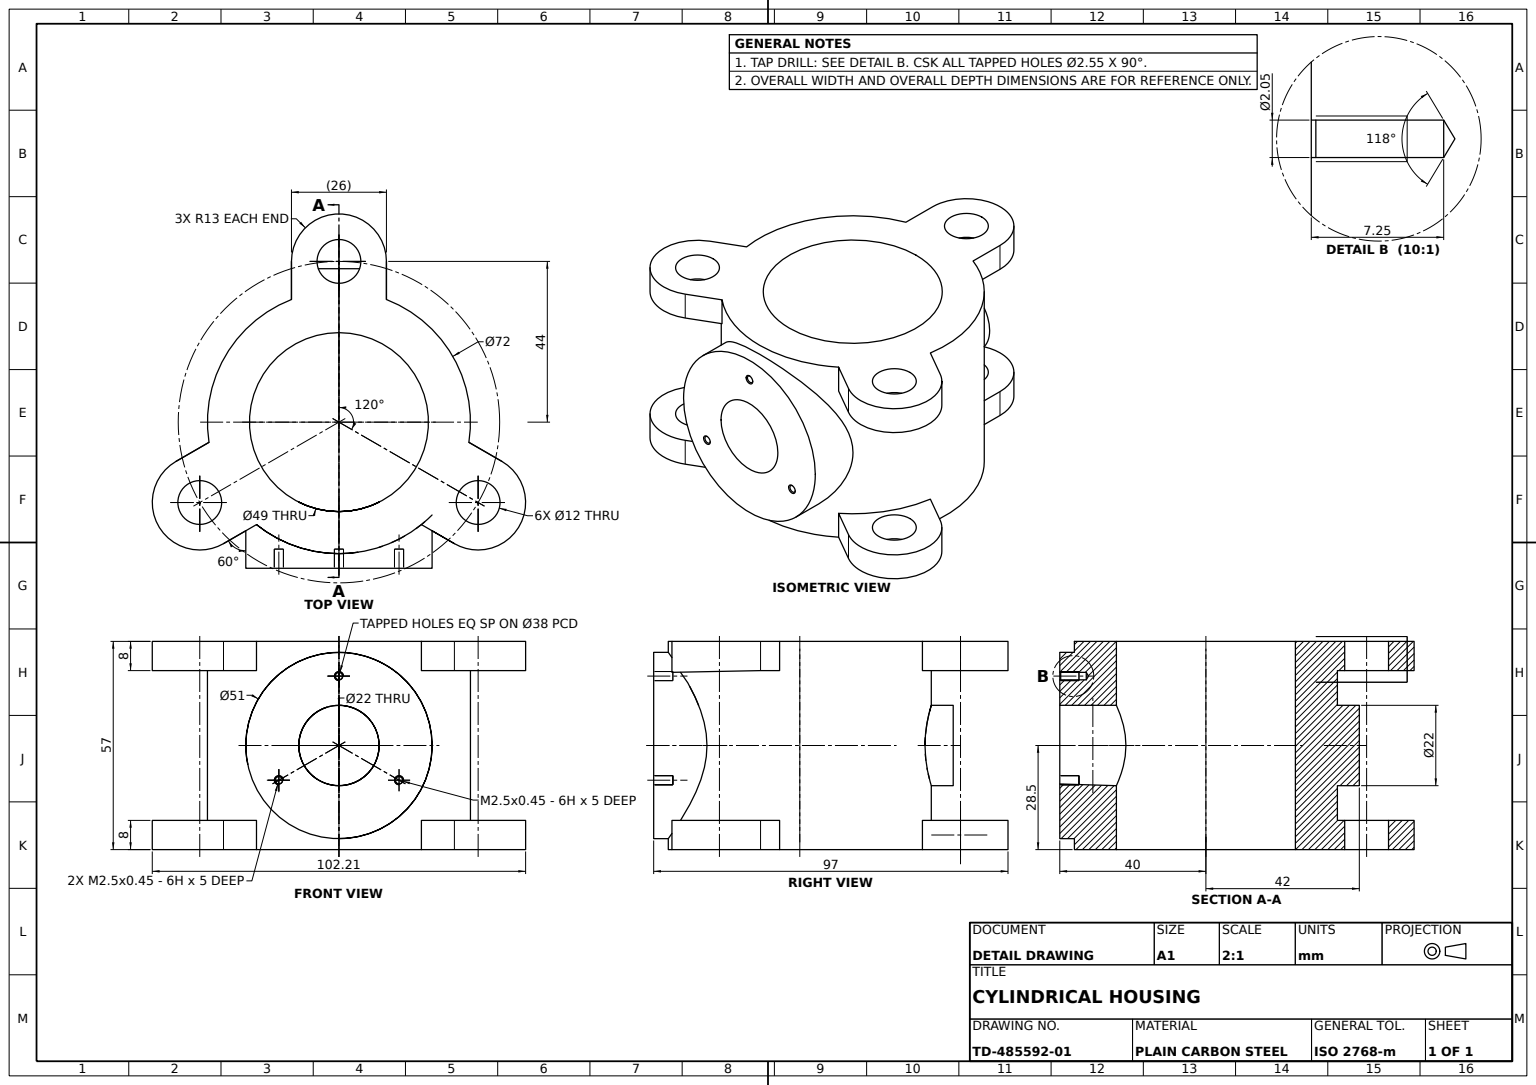
from build123d import *

# Parameters (mm, degrees)
MAIN_BODY_PROFILE_SKETCH_R             = 36
MAIN_BODY_PROFILE_SKETCH_R_2           = 24.5
MAIN_BODY_DEPTH                        = 28.5
MOUNTING_LUGS_SKETCH_R                 = 6
TOP_MOUNTING_LUGS_3X_DEPTH             = 8
SIDE_PORT_BOSS_SKETCH_51_R             = 25.5
SIDE_PORT_BOSS_51_DEPTH                = 40
PORT_TAPPED_HOLES_3XM2_5_PATTERN_COUNT = 3
MAIN_BORE_SKETCH_R                     = 24.5
MAIN_BORE_DEPTH                        = 96.444921674
SIDE_PORT_BORE_22_REACH                = 115.283
SIDE_PORT_BORE_22_END_RADIUS           = 24.5
SIDE_PORT_BORE_SKETCH_22_R             = 11
INTERNAL_BOSS_REACH                    = 102.737
INTERNAL_BOSS_END_RADIUS               = 36
INTERNAL_BOSS_SKETCH_R                 = 11


with BuildPart() as part:
    # Main Body Profile Sketch → Main Body (new, symmetric)
    with BuildSketch(Plane(origin=(0, 0, 0), x_dir=(1, 0, 0), z_dir=(0, 1, 0))):
        with Locations(Location((0, 0, 0), (0, 0, 90))):
            Circle(MAIN_BODY_PROFILE_SKETCH_R)
        with Locations(Location((0, 0, 0), (0, 0, 90))):
            Circle(MAIN_BODY_PROFILE_SKETCH_R_2, mode=Mode.SUBTRACT)
    extrude(amount=MAIN_BODY_DEPTH, both=True)

    # Mounting Lugs Sketch → Top Mounting Lugs 3x (add)
    # profile 1 of 3: a face of its own
    with BuildSketch(Plane(origin=(0, 28.5, 0), x_dir=(1, 0, 0), z_dir=(0, 1, 0))):
        with BuildLine():
            Line((-13, 44), (-13, 33.570820663))
            Line((-13, 33.570820663), (13, 33.570820663))
            Line((13, 33.570820663), (13, 44))
            ThreePointArc((13, 44), (0, 57), (-13, 44))
        make_face()
        with Locations(Location((0, 44, 0), (0, 0, 270))):
            Circle(MOUNTING_LUGS_SKETCH_R, mode=Mode.SUBTRACT)
    # profile 2 of 3: a face of its own
    with BuildSketch(Plane(origin=(0, 28.5, 0), x_dir=(1, 0, 0), z_dir=(0, 1, 0))):
        with BuildLine():
            Line((44.605117767, -10.741669751), (35.57318352, -5.527080082))
            Line((35.57318352, -5.527080082), (22.57318352, -28.043740581))
            Line((22.57318352, -28.043740581), (31.605117767, -33.258330249))
            ThreePointArc((31.605117767, -33.258330249), (49.363448016, -28.5), (44.605117767, -10.741669751))
        make_face()
        with Locations(Location((38.105117767, -22, 0), (0, 0, 270))):
            Circle(MOUNTING_LUGS_SKETCH_R, mode=Mode.SUBTRACT)
    # profile 3 of 3: a face of its own
    with BuildSketch(Plane(origin=(0, 28.5, 0), x_dir=(1, 0, 0), z_dir=(0, 1, 0))):
        with BuildLine():
            Line((-31.605117767, -33.258330249), (-22.57318352, -28.043740581))
            Line((-22.57318352, -28.043740581), (-35.57318352, -5.527080082))
            Line((-35.57318352, -5.527080082), (-44.605117767, -10.741669751))
            ThreePointArc((-44.605117767, -10.741669751), (-49.363448016, -28.5), (-31.605117767, -33.258330249))
        make_face()
        with Locations(Location((-38.105117767, -22, 0), (0, 0, 270))):
            Circle(MOUNTING_LUGS_SKETCH_R, mode=Mode.SUBTRACT)
    top_mounting_lugs_3x = extrude(amount=-TOP_MOUNTING_LUGS_3X_DEPTH)

    # Bottom Mounting Lugs Mirror: Top Mounting Lugs 3x across plane
    add(top_mounting_lugs_3x.mirror(Plane.ZX))

    # Side Port Boss Sketch Ø51 → Side Port Boss Ø51 (add)
    with BuildSketch(Plane.XY):
        with Locations(Location((0, 0, 0), (0, 0, 180))):
            Circle(SIDE_PORT_BOSS_SKETCH_51_R)
    extrude(amount=SIDE_PORT_BOSS_51_DEPTH)

    # Sketch5 → Port Tapped Hole M2.5 (revolve, cut)
    with BuildSketch(Plane(origin=(0, 19, 40), x_dir=(0, -1, 0), z_dir=(1, 0, 0))):
        Polygon((0, 0), (0, 7.865882135), (1.025, 7.25), (1.025, 0.25), (1.275, 0), align=None)
    port_tapped_hole_m2_5 = revolve(axis=Axis((0, 19, 46.35), (0, 0, -1)), mode=Mode.SUBTRACT)

    # Port Tapped Holes 3xM2.5 Pattern: Port Tapped Hole M2.5 ×3 about axis
    port_tapped_holes_3xm2_5_pattern_axis = Axis((0, 0, 0), (0, 0, 1))
    for i in range(1, PORT_TAPPED_HOLES_3XM2_5_PATTERN_COUNT):
        add(port_tapped_hole_m2_5.rotate(port_tapped_holes_3xm2_5_pattern_axis, i * 360 / PORT_TAPPED_HOLES_3XM2_5_PATTERN_COUNT), mode=Mode.SUBTRACT)

    # Main Bore Sketch → Main Bore (cut, through all)
    with BuildSketch(Plane(origin=(0, 28.5, 0), x_dir=(1, 0, 0), z_dir=(0, 1, 0))):
        with Locations(Location((0, 0, 0), (0, 0, 90))):
            Circle(MAIN_BORE_SKETCH_R)
    extrude(amount=-MAIN_BORE_DEPTH, mode=Mode.SUBTRACT)

    # Side Port Bore Ø22: up to this cylinder (the profile starts outside it)
    side_port_bore_22_end = Plane(origin=(0, 0, 0), z_dir=(0, -1, 0)) * Cylinder(SIDE_PORT_BORE_22_END_RADIUS, 280.566, mode=Mode.PRIVATE)
    # Side Port Bore Sketch Ø22 → Side Port Bore Ø22 (cut, up to the surface)
    with BuildSketch(Plane.XY.offset(40), mode=Mode.PRIVATE) as side_port_bore_22_sk1:
        Circle(SIDE_PORT_BORE_SKETCH_22_R)
    side_port_bore_22_tool1 = extrude(side_port_bore_22_sk1.sketch, amount=-SIDE_PORT_BORE_22_REACH, mode=Mode.PRIVATE) - side_port_bore_22_end
    add(side_port_bore_22_tool1.solids().sort_by_distance((0, 0, 40))[0], mode=Mode.SUBTRACT)

    # Internal Boss: up to this cylinder (the profile starts outside it)
    internal_boss_end = Plane(origin=(0, 0, 0), z_dir=(0, -1, 0)) * Cylinder(INTERNAL_BOSS_END_RADIUS, 278.474, mode=Mode.PRIVATE)
    # Internal Boss Sketch → Internal Boss (add, up to the surface)
    with BuildSketch(Plane.XY.offset(-42), mode=Mode.PRIVATE) as internal_boss_sk1:
        Circle(INTERNAL_BOSS_SKETCH_R)
    internal_boss_tool1 = extrude(internal_boss_sk1.sketch, amount=INTERNAL_BOSS_REACH, mode=Mode.PRIVATE) - internal_boss_end
    add(internal_boss_tool1.solids().sort_by_distance((0, 0, -42))[0])


solid = part.part
